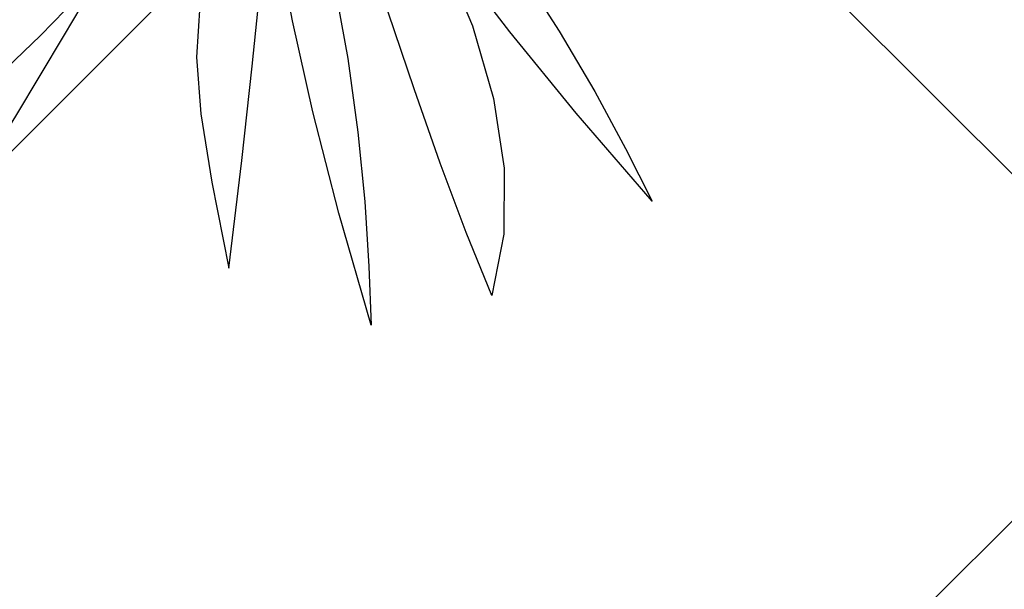
# Model space of a CAD drawing. Units: inches. Extents: x 3590 to 5167, y 65 to 1917.
# Tile 50 of 100: x 4947.17 to 4967.82, y 1503.63 to 1515.58. Entities that reach past the tile are written whole.
import ezdxf

# ---------------------------------------------------------------- set-up
doc = ezdxf.new("R2010")
doc.units = ezdxf.units.IN
doc.layers.add('A-FLOR-PATT', color=8, linetype='Continuous', lineweight=13)
doc.layers.add('L-PLNT', color=94, linetype='Continuous', lineweight=18)
doc.layers.add('DIENHOA', color=3, linetype='Continuous')

# ---------------------------------------------------------------- blocks, each defined once
blk = doc.blocks.new('Cay03_mb')
at = {"layer": 'DIENHOA'}
for p, q in [((135.85, -204.28), (162.8, -268.28)), ((-162.07, -230.91), (-206.29, -276.49)), ((113.06, -322.16), (90.79, -256.57)), ((162.8, -268.28), (180.96, -330.4)), ((-206.29, -276.49), (-249.56, -317.79)), ((135.38, -385.56), (113.06, -322.16)), ((180.96, -330.4), (190.01, -389.96)), ((157.6, -444.99), (135.38, -385.56)), ((190.01, -389.96), (189.65, -446.27)), ((179.55, -498.66), (157.6, -444.99)), ((189.65, -446.27), (179.55, -498.66))]:
    blk.add_line(p, q, dxfattribs=at)
for points in [[(23.69, -5.44), (-13.63, -87.94), (-41.14, -152.63), (-59.64, -205.04), (-69.94, -250.66), (-72.84, -295), (-69.17, -343.58), (-59.73, -401.89), (-45.32, -475.45)], [(-45.32, -475.45), (-34.09, -383.24), (-25.4, -302.82), (-18.34, -233.08), (-12.02, -172.9), (-5.55, -121.16), (1.96, -76.75), (11.41, -38.55), (23.69, -5.44)], [(316.49, -418.14), (251.44, -342.76), (194.84, -273.28), (146.52, -210.16), (106.33, -153.83), (74.11, -104.75), (49.71, -63.36), (32.95, -30.11), (23.69, -5.44)], [(23.69, -5.44), (74.94, -57.08), (121.78, -110.58), (164.32, -165.02), (202.67, -219.43), (236.95, -272.89), (267.27, -324.46), (293.75, -373.19), (316.49, -418.14)], [(-276.22, -424.43), (-227.35, -345.43), (-185.71, -276.08), (-150.05, -215.74), (-119.06, -163.76), (-91.49, -119.51), (-66.04, -82.35), (-41.43, -51.64), (-16.39, -26.73)], [(76.25, -524.2), (48.83, -428.48), (26.6, -341.67), (9.22, -264.1), (-3.63, -196.11), (-12.28, -138.04), (-17.07, -90.23), (-18.33, -53.01), (-16.39, -26.73)], [(-16.39, -26.73), (8.47, -95.11), (28.54, -163.33), (44.32, -230.59), (56.3, -296.08), (64.99, -358.99), (70.88, -418.52), (74.46, -473.86), (76.25, -524.2)]]:
    blk.add_lwpolyline(points, dxfattribs=at)

msp = doc.modelspace()

# ---------------------------------------------------------------- hatches: boundary and pattern name
at = {"layer": 'A-FLOR-PATT', "transparency": 33554687}
h = msp.add_hatch(dxfattribs=at)
h.set_pattern_fill('AR-HBONE', color=256, scale=0.2)
h.set_pattern_definition([(45, (-588.972, 0), (0, 28.73682), [60.96, -20.32]), (135, (-574.604, 14.368), (3e-15, 28.73682), [60.96, -20.32])])
h.paths.add_polyline_path([(5071.274, 1796.999), (4933.274, 1796.999), (4933.274, 1753.999), (4962.774, 1753.999, -0.414214), (4928.774, 1719.999), (4933.274, 1718.999), (4933.274, 1334.999), (5071.274, 1334.999)])
h.paths.add_polyline_path([(4951.78, 1521.077), (4951.715, 1521.04), (4951.563, 1520.895)], flags=16)
h.paths.add_polyline_path([(4952.267, 1521.376), (4952.198, 1521.371), (4952.198, 1521.356)], flags=0)
h.paths.add_polyline_path([(4967.051, 1529.728), (4965.231, 1528.694), (4963.411, 1527.714), (4961.756, 1526.851), (4963.589, 1527.449), (4964.036, 1527.478), (4962.975, 1527.249), (4961.76, 1526.852), (4959.792, 1525.834), (4958.005, 1524.895), (4956.24, 1523.93), (4954.504, 1522.919), (4954.129, 1522.682), (4953.361, 1521.997), (4953.366, 1521.998), (4953.605, 1522.064), (4955.106, 1522.761), (4956.921, 1523.434), (4958.678, 1523.915), (4960.358, 1524.2), (4961.945, 1524.286), (4964.171, 1524.108), (4965.958, 1523.309), (4963.863, 1522.976), (4965.187, 1522.499), (4963.366, 1522.497), (4961.545, 1522.487), (4959.764, 1522.461), (4958.304, 1522.419), (4957.974, 1522.388), (4956.307, 1522.232), (4954.718, 1522.071), (4953.251, 1521.899), (4953.525, 1521.623), (4954.331, 1521.379), (4956.243, 1521.23), (4958.039, 1520.93), (4959.684, 1520.483), (4961.16, 1519.896), (4963.107, 1518.8), (4964.393, 1517.325), (4962.973, 1517.726), (4964.558, 1516.661), (4965.407, 1515.708), (4963.507, 1516.322), (4961.68, 1517.005), (4959.935, 1517.745), (4958.282, 1518.528), (4956.732, 1519.343), (4955.295, 1520.175), (4954.672, 1520.572), (4954.513, 1520.627), (4955.658, 1519.318), (4956.703, 1517.982), (4957.644, 1516.647), (4958.485, 1515.334), (4959.55, 1513.524), (4960.438, 1511.769), (4958.841, 1513.62), (4957.452, 1515.325), (4955.819, 1517.459), (4956.665, 1515.448), (4957.111, 1513.923), (4957.447, 1511.714), (4957.076, 1509.793), (4956.538, 1511.11), (4955.992, 1512.569), (4955.444, 1514.125), (4954.898, 1515.735), (4954.357, 1517.356), (4953.824, 1518.943), (4953.305, 1520.452), (4953.065, 1521.116), (4952.971, 1521.146), (4952.949, 1521.086), (4952.73, 1520.199), (4953.37, 1518.024), (4953.757, 1516.373), (4954.051, 1514.765), (4954.264, 1513.221), (4954.471, 1511.131), (4954.497, 1510.402), (4954.409, 1511.76), (4954.264, 1513.221), (4954.051, 1514.765), (4953.757, 1516.373), (4953.37, 1518.024), (4952.877, 1519.698), (4952.716, 1520.141), (4952.533, 1519.059), (4952.374, 1517.789), (4952.219, 1516.312), (4952.046, 1514.6), (4951.833, 1512.626), (4951.557, 1510.363), (4951.203, 1512.168), (4950.852, 1514.339), (4950.985, 1516.376), (4951.66, 1518.286), (4952.593, 1520.481), (4952.357, 1521.13), (4951.855, 1520.328), (4950.839, 1518.908), (4949.777, 1517.587), (4948.916, 1516.617), (4948.111, 1515.256), (4947.089, 1513.554), (4945.889, 1511.615), (4946.326, 1513.402), (4946.562, 1514.249), (4945.528, 1513.327), (4944.581, 1512.531), (4946.018, 1514.508), (4947.204, 1516.048), (4947.893, 1517.313), (4949.307, 1518.764), (4950.414, 1519.767), (4950.451, 1519.806), (4952.267, 1521.376), (4951.645, 1521.493), (4950.404, 1521.18), (4948.044, 1520.359), (4946.119, 1519.452), (4944.572, 1518.475), (4943.35, 1517.443), (4941.997, 1515.92), (4941.661, 1515.275), (4942.813, 1516.99), (4944.572, 1518.475), (4946.119, 1519.452), (4948.044, 1520.359), (4950.404, 1521.18), (4951.645, 1521.493), (4949.647, 1521.868), (4948.6, 1521.756), (4947.126, 1521.57), (4945.42, 1521.348), (4943.45, 1521.105), (4941.183, 1520.856), (4942.86, 1521.613), (4943.873, 1522.03), (4942.952, 1521.909), (4941.41, 1521.485), (4939.543, 1520.67), (4938.968, 1520.226), (4940.733, 1521.299), (4942.952, 1521.909), (4943.702, 1522.008), (4945.894, 1522.7), (4947.565, 1522.714), (4948.921, 1522.566), (4951.131, 1522.183), (4950.971, 1522.297), (4948.129, 1523.006), (4946.035, 1523.707), (4944.232, 1524.521), (4942.707, 1525.461), (4941.444, 1526.537), (4940.43, 1527.761), (4939.649, 1529.143), (4941.421, 1528.122), (4943.147, 1527.132), (4944.841, 1526.175), (4946.514, 1525.25), (4948.179, 1524.359), (4948.365, 1524.263), (4946.475, 1526.045), (4945.181, 1527.54), (4944.19, 1529.033), (4943.496, 1530.54), (4943.278, 1531.36), (4942.498, 1531.919), (4943.114, 1531.762), (4942.959, 1533.659), (4944.14, 1531.989), (4944.612, 1531.323), (4946.202, 1530.463), (4947.486, 1529.509), (4948.79, 1528.226), (4950.368, 1526.237), (4949.485, 1528.155), (4948.851, 1530.123), (4948.491, 1532.041), (4948.381, 1533.918), (4948.501, 1535.76), (4948.827, 1537.573), (4949.418, 1535.565), (4949.957, 1533.569), (4950.464, 1531.586), (4950.961, 1529.617), (4951.391, 1527.954), (4951.724, 1530.687), (4952.201, 1532.58), (4952.889, 1534.33), (4953.77, 1535.951), (4954.827, 1537.46), (4954.521, 1535.39), (4954.273, 1533.937), (4955.58, 1535.663), (4956.748, 1536.739), (4956.159, 1534.78), (4955.589, 1532.873), (4955.043, 1531.006), (4954.525, 1529.166), (4954.038, 1527.341), (4953.638, 1525.733), (4953.611, 1525.586), (4953.398, 1524.166), (4953.382, 1524.009), (4954.07, 1525.476), (4954.912, 1527.022), (4956.136, 1528.894), (4957.847, 1530.577), (4959.376, 1531.54), (4958.256, 1530.104), (4957.143, 1528.663), (4956.066, 1527.243), (4955.056, 1525.871), (4954.141, 1524.571), (4953.352, 1523.372), (4953.311, 1523.303), (4953.273, 1522.925), (4953.261, 1522.382), (4954.103, 1523.373), (4954.63, 1524.284), (4955.961, 1526.358), (4957.23, 1528.13), (4958.421, 1529.609), (4960.037, 1531.368), (4961.374, 1532.375), (4962.101, 1532.77), (4961.07, 1531.061), (4959.987, 1529.438), (4958.869, 1527.908), (4958.15, 1527.007), (4959.803, 1528.003), (4961.589, 1528.793), (4963.391, 1529.328), (4965.211, 1529.632)], flags=16)
h.paths.add_polyline_path([(4962.944, 1523.182), (4961.107, 1523.422), (4960.392, 1523.362), (4962.35, 1523.331)], flags=0)
h.paths.add_polyline_path([(5049.541, 1584.551), (5049.476, 1584.515), (5049.325, 1584.37)], flags=16)
h.paths.add_polyline_path([(5050.028, 1584.851), (5049.959, 1584.845), (5049.959, 1584.83)], flags=0)
h.paths.add_polyline_path([(5042.333, 1581.949), (5043.88, 1582.926), (5045.806, 1583.833), (5048.165, 1584.654), (5049.406, 1584.967), (5047.408, 1585.342), (5046.361, 1585.231), (5044.888, 1585.044), (5043.181, 1584.822), (5041.211, 1584.579), (5038.944, 1584.33), (5040.622, 1585.087), (5041.634, 1585.504), (5040.713, 1585.383), (5039.171, 1584.959), (5037.304, 1584.144), (5036.729, 1583.7), (5038.494, 1584.773), (5040.713, 1585.383), (5041.463, 1585.482), (5043.655, 1586.174), (5045.326, 1586.188), (5046.682, 1586.04), (5048.893, 1585.657), (5048.732, 1585.771), (5045.891, 1586.48), (5043.796, 1587.181), (5041.994, 1587.996), (5040.468, 1588.935), (5039.205, 1590.011), (5038.191, 1591.235), (5037.41, 1592.617), (5039.182, 1591.596), (5040.909, 1590.607), (5042.602, 1589.649), (5044.275, 1588.724), (5045.94, 1587.833), (5046.126, 1587.738), (5044.237, 1589.519), (5042.942, 1591.015), (5041.952, 1592.508), (5041.257, 1594.014), (5041.039, 1594.834), (5040.26, 1595.393), (5040.875, 1595.237), (5040.721, 1597.133), (5041.901, 1595.463), (5042.373, 1594.798), (5043.963, 1593.938), (5045.247, 1592.983), (5046.552, 1591.701), (5048.129, 1589.712), (5047.247, 1591.63), (5046.613, 1593.597), (5046.252, 1595.515), (5046.142, 1597.392), (5046.262, 1599.234), (5046.588, 1601.047), (5047.179, 1599.039), (5047.718, 1597.043), (5048.225, 1595.06), (5048.722, 1593.091), (5049.152, 1591.429), (5049.485, 1594.161), (5049.962, 1596.054), (5050.65, 1597.804), (5051.532, 1599.425), (5052.589, 1600.934), (5052.283, 1598.864), (5052.034, 1597.411), (5053.341, 1599.137), (5054.509, 1600.213), (5053.92, 1598.254), (5053.35, 1596.348), (5052.805, 1594.48), (5052.286, 1592.64), (5051.799, 1590.815), (5051.4, 1589.207), (5051.373, 1589.06), (5051.159, 1587.64), (5051.143, 1587.483), (5051.831, 1588.95), (5052.673, 1590.496), (5053.898, 1592.368), (5055.608, 1594.051), (5057.137, 1595.014), (5056.017, 1593.578), (5054.904, 1592.137), (5053.828, 1590.717), (5052.817, 1589.345), (5051.902, 1588.046), (5051.113, 1586.846), (5051.072, 1586.777), (5051.034, 1586.399), (5051.022, 1585.856), (5051.864, 1586.847), (5052.391, 1587.758), (5053.723, 1589.832), (5054.991, 1591.604), (5056.182, 1593.083), (5057.798, 1594.842), (5059.135, 1595.849), (5059.863, 1596.244), (5058.831, 1594.535), (5057.749, 1592.912), (5056.63, 1591.382), (5055.912, 1590.482), (5057.564, 1591.477), (5059.35, 1592.267), (5061.152, 1592.802), (5062.972, 1593.106), (5064.812, 1593.203), (5062.992, 1592.169), (5061.172, 1591.188), (5059.518, 1590.325), (5061.35, 1590.924), (5061.797, 1590.952), (5060.737, 1590.723), (5059.521, 1590.326), (5057.553, 1589.308), (5055.766, 1588.369), (5054.002, 1587.404), (5052.265, 1586.393), (5051.891, 1586.156), (5051.122, 1585.471), (5051.127, 1585.472), (5051.366, 1585.538), (5052.867, 1586.235), (5054.682, 1586.908), (5056.439, 1587.389), (5058.12, 1587.675), (5059.706, 1587.76), (5061.933, 1587.583), (5063.719, 1586.783), (5061.624, 1586.45), (5062.949, 1585.973), (5061.127, 1585.971), (5059.307, 1585.961), (5057.525, 1585.935), (5056.065, 1585.893), (5055.735, 1585.862), (5054.068, 1585.707), (5052.479, 1585.546), (5051.012, 1585.373), (5051.286, 1585.097), (5052.092, 1584.853), (5054.004, 1584.704), (5055.8, 1584.404), (5057.446, 1583.958), (5058.921, 1583.37), (5060.868, 1582.274), (5062.154, 1580.799), (5060.734, 1581.2), (5062.32, 1580.135), (5063.168, 1579.182), (5061.269, 1579.796), (5059.441, 1580.479), (5057.696, 1581.219), (5056.043, 1582.003), (5054.493, 1582.817), (5053.057, 1583.649), (5052.433, 1584.047), (5052.274, 1584.101), (5053.42, 1582.793), (5054.464, 1581.457), (5055.405, 1580.121), (5056.247, 1578.809), (5057.311, 1576.998), (5058.199, 1575.244), (5056.602, 1577.094), (5055.213, 1578.799), (5053.58, 1580.933), (5054.427, 1578.922), (5054.872, 1577.397), (5055.208, 1575.189), (5054.838, 1573.267), (5054.299, 1574.584), (5053.754, 1576.043), (5053.206, 1577.599), (5052.659, 1579.209), (5052.118, 1580.83), (5051.585, 1582.417), (5051.066, 1583.927), (5050.826, 1584.59), (5050.733, 1584.62), (5050.711, 1584.561), (5050.491, 1583.673), (5051.131, 1581.498), (5051.518, 1579.847), (5051.813, 1578.24), (5052.026, 1576.695), (5052.233, 1574.605), (5052.258, 1573.876), (5052.17, 1575.234), (5052.026, 1576.695), (5051.813, 1578.24), (5051.518, 1579.847), (5051.131, 1581.498), (5050.638, 1583.172), (5050.477, 1583.615), (5050.294, 1582.533), (5050.136, 1581.263), (5049.981, 1579.786), (5049.807, 1578.074), (5049.594, 1576.1), (5049.318, 1573.837), (5048.965, 1575.642), (5048.613, 1577.813), (5048.747, 1579.85), (5049.421, 1581.76), (5050.354, 1583.955), (5050.118, 1584.604), (5049.616, 1583.802), (5048.6, 1582.382), (5047.538, 1581.061), (5046.677, 1580.091), (5045.872, 1578.73), (5044.85, 1577.028), (5043.651, 1575.089), (5044.087, 1576.877), (5044.324, 1577.723), (5043.289, 1576.801), (5042.342, 1576.005), (5043.779, 1577.982), (5044.966, 1579.522), (5045.655, 1580.787), (5047.068, 1582.239), (5048.175, 1583.241), (5048.213, 1583.28), (5050.028, 1584.851), (5049.406, 1584.967), (5048.165, 1584.654), (5045.806, 1583.833), (5043.88, 1582.926), (5042.333, 1581.949), (5041.111, 1580.917), (5039.758, 1579.394), (5039.423, 1578.749), (5040.575, 1580.464)], flags=16)
h.paths.add_polyline_path([(4954.799, 1533.12), (4954.262, 1532.079), (4953.831, 1530.935), (4953.505, 1529.636), (4953.283, 1528.133), (4953.167, 1526.376), (4953.156, 1524.315), (4953.277, 1521.236), (4952.802, 1521.842), (4951.557, 1521.998), (4950.976, 1521.961), (4952.661, 1521.941), (4952.802, 1521.842), (4953.152, 1523.593), (4953.167, 1526.376), (4953.283, 1528.133), (4953.609, 1530.346), (4954.456, 1532.592)], flags=0)
h.paths.add_polyline_path([(5050.563, 1585.316), (5049.318, 1585.472), (5048.737, 1585.435), (5050.422, 1585.415), (5050.563, 1585.316), (5050.914, 1587.067), (5050.928, 1589.851), (5051.045, 1591.607), (5051.371, 1593.82), (5052.217, 1596.066), (5052.56, 1596.594), (5052.024, 1595.554), (5051.592, 1594.409), (5051.266, 1593.11), (5051.045, 1591.607), (5050.928, 1589.851), (5050.918, 1587.789), (5051.038, 1584.71)], flags=0)
h.paths.add_polyline_path([(5058.153, 1586.836), (5060.111, 1586.805), (5060.705, 1586.656), (5058.868, 1586.896)], flags=0)
h.paths.add_polyline_path([(5049.541, 1430.936), (5049.476, 1430.9), (5049.325, 1430.755)], flags=16)
h.paths.add_polyline_path([(5050.028, 1431.236), (5049.959, 1431.231), (5049.959, 1431.215)], flags=0)
h.paths.add_polyline_path([(5046.588, 1447.432), (5047.179, 1445.425), (5047.718, 1443.429), (5048.225, 1441.446), (5048.722, 1439.476), (5049.152, 1437.814), (5049.485, 1440.546), (5049.962, 1442.439), (5050.65, 1444.189), (5051.532, 1445.811), (5052.589, 1447.319), (5052.283, 1445.249), (5052.034, 1443.796), (5053.341, 1445.522), (5054.509, 1446.598), (5053.92, 1444.64), (5053.35, 1442.733), (5052.805, 1440.865), (5052.286, 1439.025), (5051.799, 1437.201), (5051.4, 1435.592), (5051.373, 1435.445), (5051.159, 1434.025), (5051.143, 1433.868), (5051.831, 1435.335), (5052.673, 1436.881), (5053.898, 1438.753), (5055.608, 1440.436), (5057.137, 1441.4), (5056.017, 1439.963), (5054.904, 1438.522), (5053.828, 1437.102), (5052.817, 1435.73), (5051.902, 1434.431), (5051.113, 1433.231), (5051.072, 1433.162), (5051.034, 1432.784), (5051.022, 1432.242), (5051.864, 1433.232), (5052.391, 1434.143), (5053.723, 1436.217), (5054.991, 1437.989), (5056.182, 1439.468), (5057.798, 1441.227), (5059.135, 1442.235), (5059.863, 1442.629), (5058.831, 1440.921), (5057.749, 1439.298), (5056.63, 1437.767), (5055.912, 1436.867), (5057.564, 1437.863), (5059.35, 1438.652), (5061.152, 1439.187), (5062.972, 1439.491), (5064.812, 1439.588), (5062.992, 1438.554), (5061.172, 1437.573), (5059.518, 1436.71), (5061.35, 1437.309), (5061.797, 1437.337), (5060.737, 1437.108), (5059.521, 1436.711), (5057.553, 1435.693), (5055.766, 1434.754), (5054.002, 1433.789), (5052.265, 1432.778), (5051.891, 1432.541), (5051.122, 1431.856), (5051.127, 1431.857), (5051.366, 1431.923), (5052.867, 1432.62), (5054.682, 1433.293), (5056.439, 1433.775), (5058.12, 1434.06), (5059.706, 1434.145), (5061.933, 1433.968), (5063.719, 1433.168), (5061.624, 1432.835), (5062.949, 1432.358), (5061.127, 1432.357), (5059.307, 1432.346), (5057.525, 1432.32), (5056.065, 1432.278), (5055.735, 1432.248), (5054.068, 1432.092), (5052.479, 1431.931), (5051.012, 1431.759), (5051.286, 1431.482), (5052.092, 1431.238), (5054.004, 1431.089), (5055.8, 1430.789), (5057.446, 1430.343), (5058.921, 1429.755), (5060.868, 1428.66), (5062.154, 1427.185), (5060.734, 1427.585), (5062.32, 1426.52), (5063.168, 1425.567), (5061.269, 1426.181), (5059.441, 1426.865), (5057.696, 1427.604), (5056.043, 1428.388), (5054.493, 1429.202), (5053.057, 1430.034), (5052.433, 1430.432), (5052.274, 1430.487), (5053.42, 1429.178), (5054.464, 1427.842), (5055.405, 1426.506), (5056.247, 1425.194), (5057.311, 1423.383), (5058.199, 1421.629), (5056.602, 1423.479), (5055.213, 1425.184), (5053.58, 1427.318), (5054.427, 1425.307), (5054.872, 1423.782), (5055.208, 1421.574), (5054.838, 1419.652), (5054.299, 1420.97), (5053.754, 1422.428), (5053.206, 1423.984), (5052.659, 1425.595), (5052.118, 1427.215), (5051.585, 1428.802), (5051.066, 1430.312), (5050.826, 1430.975), (5050.733, 1431.005), (5050.711, 1430.946), (5050.491, 1430.058), (5051.131, 1427.883), (5051.518, 1426.232), (5051.813, 1424.625), (5052.026, 1423.081), (5052.233, 1420.991), (5052.258, 1420.261), (5052.17, 1421.619), (5052.026, 1423.081), (5051.813, 1424.625), (5051.518, 1426.232), (5051.131, 1427.883), (5050.638, 1429.558), (5050.477, 1430.001), (5050.294, 1428.918), (5050.136, 1427.648), (5049.981, 1426.171), (5049.807, 1424.459), (5049.594, 1422.485), (5049.318, 1420.222), (5048.965, 1422.028), (5048.613, 1424.199), (5048.747, 1426.235), (5049.421, 1428.146), (5050.354, 1430.34), (5050.118, 1430.989), (5049.616, 1430.187), (5048.6, 1428.768), (5047.538, 1427.446), (5046.677, 1426.477), (5045.872, 1425.116), (5044.85, 1423.413), (5043.651, 1421.474), (5044.087, 1423.262), (5044.324, 1424.109), (5043.289, 1423.186), (5042.342, 1422.391), (5043.779, 1424.368), (5044.966, 1425.907), (5045.655, 1427.173), (5047.068, 1428.624), (5048.175, 1429.627), (5048.213, 1429.666), (5050.028, 1431.236), (5049.406, 1431.353), (5048.165, 1431.039), (5045.806, 1430.218), (5043.88, 1429.311), (5042.333, 1428.334), (5041.111, 1427.302), (5039.758, 1425.779), (5039.423, 1425.134), (5040.575, 1426.849), (5042.333, 1428.334), (5043.88, 1429.311), (5045.806, 1430.218), (5048.165, 1431.039), (5049.406, 1431.353), (5047.408, 1431.727), (5046.361, 1431.616), (5044.888, 1431.429), (5043.181, 1431.207), (5041.211, 1430.964), (5038.944, 1430.715), (5040.622, 1431.472), (5041.634, 1431.89), (5040.713, 1431.769), (5039.171, 1431.345), (5037.304, 1430.53), (5036.729, 1430.085), (5038.494, 1431.158), (5040.713, 1431.769), (5041.463, 1431.867), (5043.655, 1432.559), (5045.326, 1432.573), (5046.682, 1432.425), (5048.893, 1432.042), (5048.732, 1432.156), (5045.891, 1432.865), (5043.796, 1433.566), (5041.994, 1434.381), (5040.468, 1435.321), (5039.205, 1436.396), (5038.191, 1437.62), (5037.41, 1439.002), (5039.182, 1437.982), (5040.909, 1436.992), (5042.602, 1436.034), (5044.275, 1435.109), (5045.94, 1434.218), (5046.126, 1434.123), (5044.237, 1435.904), (5042.942, 1437.4), (5041.952, 1438.893), (5041.257, 1440.399), (5041.039, 1441.219), (5040.26, 1441.778), (5040.875, 1441.622), (5040.721, 1443.518), (5041.901, 1441.848), (5042.373, 1441.183), (5043.963, 1440.323), (5045.247, 1439.369), (5046.552, 1438.086), (5048.129, 1436.097), (5047.247, 1438.015), (5046.613, 1439.982), (5046.252, 1441.901), (5046.142, 1443.778), (5046.262, 1445.619)], flags=16)
h.paths.add_polyline_path([(5052.382, 1444.255), (5051.623, 1442.78), (5052.024, 1441.939), (5052.56, 1442.98)], flags=0)
h.paths.add_polyline_path([(5050.563, 1431.701), (5049.318, 1431.857), (5048.737, 1431.821), (5050.422, 1431.8)], flags=0)
h.paths.add_polyline_path([(5058.153, 1433.221), (5060.111, 1433.19), (5060.705, 1433.041), (5058.868, 1433.281)], flags=0)
h.paths.add_polyline_path([(5049.541, 1352.285), (5049.476, 1352.249), (5049.325, 1352.104)], flags=16)
h.paths.add_polyline_path([(5050.028, 1352.585), (5049.959, 1352.58), (5049.959, 1352.564)], flags=0)
h.paths.add_polyline_path([(5046.588, 1368.781), (5047.179, 1366.774), (5047.718, 1364.778), (5048.225, 1362.795), (5048.722, 1360.825), (5049.152, 1359.163), (5049.485, 1361.896), (5049.962, 1363.789), (5050.65, 1365.538), (5051.532, 1367.16), (5052.589, 1368.669), (5052.283, 1366.598), (5052.034, 1365.145), (5053.341, 1366.871), (5054.509, 1367.947), (5053.92, 1365.989), (5053.35, 1364.082), (5052.805, 1362.214), (5052.286, 1360.374), (5051.799, 1358.55), (5051.4, 1356.942), (5051.373, 1356.794), (5051.159, 1355.374), (5051.143, 1355.218), (5051.831, 1356.684), (5052.673, 1358.23), (5053.898, 1360.102), (5055.608, 1361.786), (5057.137, 1362.749), (5056.017, 1361.313), (5054.904, 1359.872), (5053.828, 1358.452), (5052.817, 1357.079), (5051.902, 1355.78), (5051.113, 1354.581), (5051.072, 1354.512), (5051.034, 1354.133), (5051.022, 1353.591), (5051.864, 1354.581), (5052.391, 1355.492), (5053.723, 1357.566), (5054.991, 1359.338), (5056.182, 1360.817), (5057.798, 1362.577), (5059.135, 1363.584), (5059.863, 1363.979), (5058.831, 1362.27), (5057.749, 1360.647), (5056.63, 1359.117), (5055.912, 1358.216), (5057.564, 1359.212), (5059.35, 1360.001), (5061.152, 1360.536), (5062.972, 1360.841), (5064.812, 1360.937), (5062.992, 1359.903), (5061.172, 1358.923), (5059.518, 1358.059), (5061.35, 1358.658), (5061.797, 1358.687), (5060.737, 1358.458), (5059.521, 1358.061), (5057.553, 1357.043), (5055.766, 1356.103), (5054.002, 1355.138), (5052.265, 1354.127), (5051.891, 1353.89), (5051.122, 1353.206), (5051.127, 1353.206), (5051.366, 1353.272), (5052.867, 1353.969), (5054.682, 1354.643), (5056.439, 1355.124), (5058.12, 1355.409), (5059.706, 1355.495), (5061.933, 1355.317), (5063.719, 1354.518), (5061.624, 1354.184), (5062.949, 1353.708), (5061.127, 1353.706), (5059.307, 1353.695), (5057.525, 1353.669), (5056.065, 1353.627), (5055.735, 1353.597), (5054.068, 1353.441), (5052.479, 1353.28), (5051.012, 1353.108), (5051.286, 1352.831), (5052.092, 1352.587), (5054.004, 1352.439), (5055.8, 1352.138), (5057.446, 1351.692), (5058.921, 1351.104), (5060.868, 1350.009), (5062.154, 1348.534), (5060.734, 1348.935), (5062.32, 1347.869), (5063.168, 1346.916), (5061.269, 1347.53), (5059.441, 1348.214), (5057.696, 1348.954), (5056.043, 1349.737), (5054.493, 1350.551), (5053.057, 1351.383), (5052.433, 1351.781), (5052.274, 1351.836), (5053.42, 1350.527), (5054.464, 1349.191), (5055.405, 1347.855), (5056.247, 1346.543), (5057.311, 1344.733), (5058.199, 1342.978), (5056.602, 1344.828), (5055.213, 1346.534), (5053.58, 1348.667), (5054.427, 1346.656), (5054.872, 1345.132), (5055.208, 1342.923), (5054.838, 1341.002), (5054.299, 1342.319), (5053.754, 1343.778), (5053.206, 1345.334), (5052.659, 1346.944), (5052.118, 1348.564), (5051.585, 1350.151), (5051.066, 1351.661), (5050.826, 1352.324), (5050.733, 1352.355), (5050.711, 1352.295), (5050.491, 1351.408), (5051.131, 1349.232), (5051.518, 1347.581), (5051.813, 1345.974), (5052.026, 1344.43), (5052.233, 1342.34), (5052.258, 1341.61), (5052.17, 1342.969), (5052.026, 1344.43), (5051.813, 1345.974), (5051.518, 1347.581), (5051.131, 1349.232), (5050.638, 1350.907), (5050.477, 1351.35), (5050.294, 1350.267), (5050.136, 1348.997), (5049.981, 1347.52), (5049.807, 1345.809), (5049.594, 1343.835), (5049.318, 1341.571), (5048.965, 1343.377), (5048.613, 1345.548), (5048.747, 1347.585), (5049.421, 1349.495), (5050.354, 1351.689), (5050.118, 1352.339), (5049.616, 1351.536), (5048.6, 1350.117), (5047.538, 1348.795), (5046.677, 1347.826), (5045.872, 1346.465), (5044.85, 1344.763), (5043.651, 1342.824), (5044.087, 1344.611), (5044.324, 1345.458), (5043.289, 1344.535), (5042.342, 1343.74), (5043.779, 1345.717), (5044.966, 1347.256), (5045.655, 1348.522), (5047.068, 1349.973), (5048.175, 1350.976), (5048.213, 1351.015), (5050.028, 1352.585), (5049.406, 1352.702), (5048.165, 1352.388), (5045.806, 1351.567), (5043.88, 1350.661), (5042.333, 1349.683), (5041.111, 1348.651), (5039.758, 1347.128), (5039.423, 1346.483), (5040.575, 1348.198), (5042.333, 1349.683), (5043.88, 1350.661), (5045.806, 1351.567), (5048.165, 1352.388), (5049.406, 1352.702), (5047.408, 1353.076), (5046.361, 1352.965), (5044.888, 1352.779), (5043.181, 1352.556), (5041.211, 1352.313), (5038.944, 1352.065), (5040.622, 1352.821), (5041.634, 1353.239), (5040.713, 1353.118), (5039.171, 1352.694), (5037.304, 1351.879), (5036.729, 1351.434), (5038.494, 1352.508), (5040.713, 1353.118), (5041.463, 1353.216), (5043.655, 1353.909), (5045.326, 1353.923), (5046.682, 1353.774), (5048.893, 1353.391), (5048.732, 1353.506), (5045.891, 1354.214), (5043.796, 1354.915), (5041.994, 1355.73), (5040.468, 1356.67), (5039.205, 1357.746), (5038.191, 1358.969), (5037.41, 1360.352), (5039.182, 1359.331), (5040.909, 1358.341), (5042.602, 1357.383), (5044.275, 1356.458), (5045.94, 1355.567), (5046.126, 1355.472), (5044.237, 1357.253), (5042.942, 1358.749), (5041.952, 1360.242), (5041.257, 1361.748), (5041.039, 1362.568), (5040.26, 1363.128), (5040.875, 1362.971), (5040.721, 1364.867), (5041.901, 1363.197), (5042.373, 1362.532), (5043.963, 1361.672), (5045.247, 1360.718), (5046.552, 1359.435), (5048.129, 1357.446), (5047.247, 1359.364), (5046.613, 1361.331), (5046.252, 1363.25), (5046.142, 1365.127), (5046.262, 1366.969)], flags=16)
h.paths.add_polyline_path([(5052.382, 1365.604), (5051.623, 1364.129), (5052.024, 1363.288), (5052.56, 1364.329)], flags=0)
h.paths.add_polyline_path([(4951.78, 1698.041), (4951.715, 1698.005), (4951.563, 1697.859)], flags=16)
h.paths.add_polyline_path([(4952.267, 1698.341), (4952.198, 1698.335), (4952.198, 1698.32)], flags=0)
h.paths.add_polyline_path([(4957.076, 1686.757), (4956.538, 1688.074), (4955.992, 1689.533), (4955.444, 1691.089), (4954.898, 1692.699), (4954.357, 1694.32), (4953.824, 1695.907), (4953.305, 1697.417), (4953.065, 1698.08), (4952.971, 1698.11), (4952.949, 1698.051), (4952.73, 1697.163), (4953.37, 1694.988), (4953.757, 1693.337), (4954.051, 1691.729), (4954.264, 1690.185), (4954.471, 1688.095), (4954.497, 1687.366), (4954.409, 1688.724), (4954.264, 1690.185), (4954.051, 1691.729), (4953.757, 1693.337), (4953.37, 1694.988), (4952.877, 1696.662), (4952.716, 1697.105), (4952.533, 1696.023), (4952.374, 1694.753), (4952.219, 1693.276), (4952.046, 1691.564), (4951.833, 1689.59), (4951.557, 1687.327), (4951.203, 1689.132), (4950.852, 1691.303), (4950.985, 1693.34), (4951.66, 1695.25), (4952.593, 1697.445), (4952.357, 1698.094), (4951.855, 1697.292), (4950.839, 1695.872), (4949.777, 1694.551), (4948.916, 1693.581), (4948.111, 1692.22), (4947.089, 1690.518), (4945.889, 1688.579), (4946.326, 1690.366), (4946.562, 1691.213), (4945.528, 1690.291), (4944.581, 1689.495), (4946.018, 1691.472), (4947.204, 1693.012), (4947.893, 1694.277), (4949.307, 1695.729), (4950.414, 1696.731), (4950.451, 1696.77), (4952.267, 1698.341), (4951.645, 1698.457), (4950.404, 1698.144), (4948.044, 1697.323), (4946.119, 1696.416), (4944.572, 1695.439), (4943.35, 1694.407), (4941.997, 1692.884), (4941.661, 1692.239), (4942.813, 1693.954), (4944.572, 1695.439), (4946.119, 1696.416), (4948.044, 1697.323), (4950.404, 1698.144), (4951.645, 1698.457), (4949.647, 1698.832), (4948.6, 1698.72), (4947.126, 1698.534), (4945.42, 1698.312), (4943.45, 1698.069), (4941.183, 1697.82), (4942.86, 1698.577), (4943.873, 1698.994), (4942.952, 1698.873), (4941.41, 1698.449), (4939.543, 1697.634), (4938.968, 1697.19), (4940.733, 1698.263), (4942.952, 1698.873), (4943.702, 1698.972), (4945.894, 1699.664), (4947.565, 1699.678), (4948.921, 1699.53), (4951.131, 1699.147), (4950.971, 1699.261), (4948.129, 1699.97), (4946.035, 1700.671), (4944.232, 1701.486), (4942.707, 1702.425), (4941.444, 1703.501), (4940.43, 1704.725), (4939.649, 1706.107), (4941.421, 1705.086), (4943.147, 1704.097), (4944.841, 1703.139), (4946.514, 1702.214), (4948.179, 1701.323), (4948.365, 1701.227), (4946.475, 1703.009), (4945.181, 1704.505), (4944.19, 1705.997), (4943.496, 1707.504), (4943.278, 1708.324), (4942.498, 1708.883), (4943.114, 1708.727), (4942.959, 1710.623), (4944.14, 1708.953), (4944.612, 1708.287), (4946.202, 1707.428), (4947.486, 1706.473), (4948.79, 1705.191), (4950.368, 1703.202), (4949.485, 1705.12), (4948.851, 1707.087), (4948.491, 1709.005), (4948.381, 1710.882), (4948.501, 1712.724), (4948.827, 1714.537), (4949.418, 1712.529), (4949.957, 1710.533), (4950.464, 1708.55), (4950.961, 1706.581), (4951.391, 1704.919), (4951.724, 1707.651), (4952.201, 1709.544), (4952.889, 1711.294), (4953.77, 1712.915), (4954.827, 1714.424), (4954.521, 1712.354), (4954.273, 1710.901), (4955.58, 1712.627), (4956.748, 1713.703), (4956.159, 1711.744), (4955.589, 1709.837), (4955.043, 1707.97), (4954.525, 1706.13), (4954.038, 1704.305), (4953.638, 1702.697), (4953.611, 1702.55), (4953.398, 1701.13), (4953.382, 1700.973), (4954.07, 1702.44), (4954.912, 1703.986), (4956.136, 1705.858), (4957.847, 1707.541), (4959.376, 1708.504), (4958.256, 1707.068), (4957.143, 1705.627), (4956.066, 1704.207), (4955.056, 1702.835), (4954.141, 1701.536), (4953.352, 1700.336), (4953.311, 1700.267), (4953.273, 1699.889), (4953.261, 1699.346), (4954.103, 1700.337), (4954.63, 1701.248), (4955.961, 1703.322), (4957.23, 1705.094), (4958.421, 1706.573), (4960.037, 1708.332), (4961.374, 1709.339), (4962.101, 1709.734), (4961.07, 1708.025), (4959.987, 1706.402), (4958.869, 1704.872), (4958.15, 1703.972), (4959.803, 1704.967), (4961.589, 1705.757), (4963.391, 1706.292), (4965.211, 1706.596), (4967.051, 1706.692), (4965.231, 1705.659), (4963.411, 1704.678), (4961.756, 1703.815), (4963.589, 1704.413), (4964.036, 1704.442), (4962.975, 1704.213), (4961.76, 1703.816), (4959.792, 1702.798), (4958.005, 1701.859), (4956.24, 1700.894), (4954.504, 1699.883), (4954.129, 1699.646), (4953.361, 1698.961), (4953.366, 1698.962), (4953.605, 1699.028), (4955.106, 1699.725), (4956.921, 1700.398), (4958.678, 1700.879), (4960.358, 1701.164), (4961.945, 1701.25), (4964.171, 1701.073), (4965.958, 1700.273), (4963.863, 1699.94), (4965.187, 1699.463), (4963.366, 1699.461), (4961.545, 1699.451), (4959.764, 1699.425), (4958.304, 1699.383), (4957.974, 1699.352), (4956.307, 1699.197), (4954.718, 1699.036), (4953.251, 1698.863), (4953.525, 1698.587), (4954.331, 1698.343), (4956.243, 1698.194), (4958.039, 1697.894), (4959.684, 1697.447), (4961.16, 1696.86), (4963.107, 1695.764), (4964.393, 1694.289), (4962.973, 1694.69), (4964.558, 1693.625), (4965.407, 1692.672), (4963.507, 1693.286), (4961.68, 1693.969), (4959.935, 1694.709), (4958.282, 1695.492), (4956.732, 1696.307), (4955.295, 1697.139), (4954.672, 1697.536), (4954.513, 1697.591), (4955.658, 1696.282), (4956.703, 1694.946), (4957.644, 1693.611), (4958.485, 1692.298), (4959.55, 1690.488), (4960.438, 1688.733), (4958.841, 1690.584), (4957.452, 1692.289), (4955.819, 1694.423), (4956.665, 1692.412), (4957.111, 1690.887), (4957.447, 1688.678)], flags=16)
h.paths.add_polyline_path([(5050.563, 1353.05), (5049.318, 1353.207), (5048.737, 1353.17), (5050.422, 1353.15)], flags=0)
h.paths.add_polyline_path([(4951.78, 1351.486), (4951.715, 1351.45), (4951.563, 1351.305)], flags=16)
h.paths.add_polyline_path([(4952.267, 1351.786), (4952.198, 1351.78), (4952.198, 1351.765)], flags=0)
h.paths.add_polyline_path([(4954.827, 1367.869), (4954.521, 1365.799), (4954.273, 1364.346), (4955.58, 1366.072), (4956.748, 1367.148), (4956.159, 1365.19), (4955.589, 1363.283), (4955.043, 1361.415), (4954.525, 1359.575), (4954.038, 1357.751), (4953.638, 1356.142), (4953.611, 1355.995), (4953.398, 1354.575), (4953.382, 1354.418), (4954.07, 1355.885), (4954.912, 1357.431), (4956.136, 1359.303), (4957.847, 1360.986), (4959.376, 1361.95), (4958.256, 1360.513), (4957.143, 1359.072), (4956.066, 1357.652), (4955.056, 1356.28), (4954.141, 1354.981), (4953.352, 1353.781), (4953.311, 1353.712), (4953.273, 1353.334), (4953.261, 1352.792), (4954.103, 1353.782), (4954.63, 1354.693), (4955.961, 1356.767), (4957.23, 1358.539), (4958.421, 1360.018), (4960.037, 1361.777), (4961.374, 1362.785), (4962.101, 1363.179), (4961.07, 1361.471), (4959.987, 1359.848), (4958.869, 1358.317), (4958.15, 1357.417), (4959.803, 1358.413), (4961.589, 1359.202), (4963.391, 1359.737), (4965.211, 1360.041), (4967.051, 1360.138), (4965.231, 1359.104), (4963.411, 1358.123), (4961.756, 1357.26), (4963.589, 1357.859), (4964.036, 1357.887), (4962.975, 1357.658), (4961.76, 1357.261), (4959.792, 1356.243), (4958.005, 1355.304), (4956.24, 1354.339), (4954.504, 1353.328), (4954.129, 1353.091), (4953.361, 1352.406), (4953.366, 1352.407), (4953.605, 1352.473), (4955.106, 1353.17), (4956.921, 1353.843), (4958.678, 1354.325), (4960.358, 1354.61), (4961.945, 1354.695), (4964.171, 1354.518), (4965.958, 1353.718), (4963.863, 1353.385), (4965.187, 1352.908), (4963.366, 1352.907), (4961.545, 1352.896), (4959.764, 1352.87), (4958.304, 1352.828), (4957.974, 1352.798), (4956.307, 1352.642), (4954.718, 1352.481), (4953.251, 1352.309), (4953.525, 1352.032), (4954.331, 1351.788), (4956.243, 1351.639), (4958.039, 1351.339), (4959.684, 1350.893), (4961.16, 1350.305), (4963.107, 1349.21), (4964.393, 1347.735), (4962.973, 1348.135), (4964.558, 1347.07), (4965.407, 1346.117), (4963.507, 1346.731), (4961.68, 1347.414), (4959.935, 1348.154), (4958.282, 1348.938), (4956.732, 1349.752), (4955.295, 1350.584), (4954.672, 1350.982), (4954.513, 1351.036), (4955.658, 1349.728), (4956.703, 1348.392), (4957.644, 1347.056), (4958.485, 1345.744), (4959.55, 1343.933), (4960.438, 1342.179), (4958.841, 1344.029), (4957.452, 1345.734), (4955.819, 1347.868), (4956.665, 1345.857), (4957.111, 1344.332), (4957.447, 1342.124), (4957.076, 1340.202), (4956.538, 1341.52), (4955.992, 1342.978), (4955.444, 1344.534), (4954.898, 1346.145), (4954.357, 1347.765), (4953.824, 1349.352), (4953.305, 1350.862), (4953.065, 1351.525), (4952.971, 1351.555), (4952.949, 1351.496), (4952.73, 1350.608), (4953.37, 1348.433), (4953.757, 1346.782), (4954.051, 1345.175), (4954.264, 1343.631), (4954.471, 1341.541), (4954.497, 1340.811), (4954.409, 1342.169), (4954.264, 1343.631), (4954.051, 1345.175), (4953.757, 1346.782), (4953.37, 1348.433), (4952.877, 1350.108), (4952.716, 1350.551), (4952.533, 1349.468), (4952.374, 1348.198), (4952.219, 1346.721), (4952.046, 1345.009), (4951.833, 1343.035), (4951.557, 1340.772), (4951.203, 1342.578), (4950.852, 1344.749), (4950.985, 1346.785), (4951.66, 1348.696), (4952.593, 1350.89), (4952.357, 1351.539), (4951.855, 1350.737), (4950.839, 1349.318), (4949.777, 1347.996), (4948.916, 1347.027), (4948.111, 1345.665), (4947.089, 1343.963), (4945.889, 1342.024), (4946.326, 1343.812), (4946.562, 1344.659), (4945.528, 1343.736), (4944.581, 1342.941), (4946.018, 1344.918), (4947.204, 1346.457), (4947.893, 1347.723), (4949.307, 1349.174), (4950.414, 1350.177), (4950.451, 1350.216), (4952.267, 1351.786), (4951.645, 1351.903), (4950.404, 1351.589), (4948.044, 1350.768), (4946.119, 1349.861), (4944.572, 1348.884), (4943.35, 1347.852), (4941.997, 1346.329), (4941.661, 1345.684), (4942.813, 1347.399), (4944.572, 1348.884), (4946.119, 1349.861), (4948.044, 1350.768), (4950.404, 1351.589), (4951.645, 1351.903), (4949.647, 1352.277), (4948.6, 1352.166), (4947.126, 1351.979), (4945.42, 1351.757), (4943.45, 1351.514), (4941.183, 1351.265), (4942.86, 1352.022), (4943.873, 1352.44), (4942.952, 1352.319), (4941.41, 1351.895), (4939.543, 1351.08), (4938.968, 1350.635), (4940.733, 1351.708), (4942.952, 1352.319), (4943.702, 1352.417), (4945.894, 1353.109), (4947.565, 1353.123), (4948.921, 1352.975), (4951.131, 1352.592), (4950.971, 1352.706), (4948.129, 1353.415), (4946.035, 1354.116), (4944.232, 1354.931), (4942.707, 1355.871), (4941.444, 1356.946), (4940.43, 1358.17), (4939.649, 1359.552), (4941.421, 1358.532), (4943.147, 1357.542), (4944.841, 1356.584), (4946.514, 1355.659), (4948.179, 1354.768), (4948.365, 1354.673), (4946.475, 1356.454), (4945.181, 1357.95), (4944.19, 1359.443), (4943.496, 1360.949), (4943.278, 1361.769), (4942.498, 1362.328), (4943.114, 1362.172), (4942.959, 1364.068), (4944.14, 1362.398), (4944.612, 1361.733), (4946.202, 1360.873), (4947.486, 1359.919), (4948.79, 1358.636), (4950.368, 1356.647), (4949.485, 1358.565), (4948.851, 1360.532), (4948.491, 1362.451), (4948.381, 1364.328), (4948.501, 1366.169), (4948.827, 1367.982), (4949.418, 1365.975), (4949.957, 1363.979), (4950.464, 1361.995), (4950.961, 1360.026), (4951.391, 1358.364), (4951.724, 1361.096), (4952.201, 1362.989), (4952.889, 1364.739), (4953.77, 1366.361)], flags=16)
h.paths.add_polyline_path([(4954.799, 1363.53), (4954.262, 1362.489), (4953.831, 1361.344), (4953.505, 1360.045), (4953.283, 1358.543), (4953.167, 1356.786), (4953.156, 1354.724), (4953.277, 1351.646), (4952.802, 1352.251), (4951.557, 1352.407), (4950.976, 1352.371), (4952.661, 1352.35), (4952.802, 1352.251), (4953.152, 1354.002), (4953.167, 1356.786), (4953.283, 1358.543), (4953.609, 1360.755), (4954.456, 1363.001)], flags=0)
h.paths.add_polyline_path([(4952.802, 1698.806), (4951.557, 1698.962), (4950.976, 1698.925), (4952.661, 1698.905), (4952.802, 1698.806), (4953.152, 1700.557), (4953.167, 1703.34), (4953.283, 1705.097), (4953.609, 1707.31), (4954.456, 1709.556), (4954.799, 1710.084), (4954.262, 1709.043), (4953.831, 1707.899), (4953.505, 1706.6), (4953.283, 1705.097), (4953.167, 1703.34), (4953.156, 1701.279), (4953.277, 1698.2)], flags=0)
h.paths.add_polyline_path([(4962.944, 1700.146), (4961.107, 1700.386), (4960.392, 1700.326), (4962.35, 1700.295)], flags=0)
h.paths.add_polyline_path([(5058.153, 1354.57), (5060.111, 1354.539), (5060.705, 1354.391), (5058.868, 1354.631)], flags=0)
h.paths.add_polyline_path([(4962.944, 1353.591), (4961.107, 1353.831), (4960.392, 1353.771), (4962.35, 1353.74)], flags=0)
h.paths.add_polyline_path([(5049.541, 1778.72), (5049.476, 1778.684), (5049.325, 1778.539)], flags=16)
h.paths.add_polyline_path([(5050.028, 1779.02), (5049.959, 1779.014), (5049.959, 1778.999)], flags=0)
h.paths.add_polyline_path([(5052.258, 1768.045), (5052.17, 1769.403), (5052.026, 1770.864), (5051.813, 1772.409), (5051.518, 1774.016), (5051.131, 1775.667), (5050.638, 1777.341), (5050.477, 1777.784), (5050.294, 1776.702), (5050.136, 1775.432), (5049.981, 1773.955), (5049.807, 1772.243), (5049.594, 1770.269), (5049.318, 1768.006), (5048.965, 1769.811), (5048.613, 1771.982), (5048.747, 1774.019), (5049.421, 1775.929), (5050.354, 1778.124), (5050.118, 1778.773), (5049.616, 1777.971), (5048.6, 1776.551), (5047.538, 1775.23), (5046.677, 1774.26), (5045.872, 1772.899), (5044.85, 1771.197), (5043.651, 1769.258), (5044.087, 1771.046), (5044.324, 1771.892), (5043.289, 1770.97), (5042.342, 1770.174), (5043.779, 1772.151), (5044.966, 1773.691), (5045.655, 1774.956), (5047.068, 1776.408), (5048.175, 1777.41), (5048.213, 1777.449), (5050.028, 1779.02), (5049.406, 1779.136), (5048.165, 1778.823), (5045.806, 1778.002), (5043.88, 1777.095), (5042.333, 1776.118), (5041.111, 1775.086), (5039.758, 1773.563), (5039.423, 1772.918), (5040.575, 1774.633), (5042.333, 1776.118), (5043.88, 1777.095), (5045.806, 1778.002), (5048.165, 1778.823), (5049.406, 1779.136), (5047.408, 1779.511), (5046.361, 1779.4), (5044.888, 1779.213), (5043.181, 1778.991), (5041.211, 1778.748), (5038.944, 1778.499), (5040.622, 1779.256), (5041.634, 1779.673), (5040.713, 1779.552), (5039.171, 1779.128), (5037.304, 1778.313), (5036.729, 1777.869), (5038.494, 1778.942), (5040.713, 1779.552), (5041.463, 1779.651), (5043.655, 1780.343), (5045.326, 1780.357), (5046.682, 1780.209), (5048.893, 1779.826), (5048.732, 1779.94), (5045.891, 1780.649), (5043.796, 1781.35), (5041.994, 1782.165), (5040.468, 1783.104), (5039.205, 1784.18), (5038.191, 1785.404), (5037.41, 1786.786), (5039.182, 1785.765), (5040.909, 1784.776), (5042.602, 1783.818), (5044.275, 1782.893), (5045.94, 1782.002), (5046.126, 1781.907), (5044.237, 1783.688), (5042.942, 1785.184), (5041.952, 1786.677), (5041.257, 1788.183), (5041.039, 1789.003), (5040.26, 1789.562), (5040.875, 1789.406), (5040.721, 1791.302), (5041.901, 1789.632), (5042.373, 1788.967), (5043.963, 1788.107), (5045.247, 1787.152), (5046.552, 1785.87), (5048.129, 1783.881), (5047.247, 1785.799), (5046.613, 1787.766), (5046.252, 1789.684), (5046.142, 1791.561), (5046.262, 1793.403), (5046.588, 1795.216), (5047.179, 1793.208), (5047.718, 1791.213), (5048.225, 1789.229), (5048.722, 1787.26), (5049.152, 1785.598), (5049.485, 1788.33), (5049.962, 1790.223), (5050.65, 1791.973), (5051.532, 1793.594), (5052.589, 1795.103), (5052.283, 1793.033), (5052.034, 1791.58), (5053.341, 1793.306), (5054.509, 1794.382), (5053.92, 1792.423), (5053.35, 1790.517), (5052.805, 1788.649), (5052.286, 1786.809), (5051.799, 1784.984), (5051.4, 1783.376), (5051.373, 1783.229), (5051.159, 1781.809), (5051.143, 1781.652), (5051.831, 1783.119), (5052.673, 1784.665), (5053.898, 1786.537), (5055.608, 1788.22), (5057.137, 1789.183), (5056.017, 1787.747), (5054.904, 1786.306), (5053.828, 1784.886), (5052.817, 1783.514), (5051.902, 1782.215), (5051.113, 1781.015), (5051.072, 1780.946), (5051.034, 1780.568), (5051.022, 1780.025), (5051.864, 1781.016), (5052.391, 1781.927), (5053.723, 1784.001), (5054.991, 1785.773), (5056.182, 1787.252), (5057.798, 1789.011), (5059.135, 1790.018), (5059.863, 1790.413), (5058.831, 1788.704), (5057.749, 1787.081), (5056.63, 1785.551), (5055.912, 1784.651), (5057.564, 1785.646), (5059.35, 1786.436), (5061.152, 1786.971), (5062.972, 1787.275), (5064.812, 1787.372), (5062.992, 1786.338), (5061.172, 1785.357), (5059.518, 1784.494), (5061.35, 1785.093), (5061.797, 1785.121), (5060.737, 1784.892), (5059.521, 1784.495), (5057.553, 1783.477), (5055.766, 1782.538), (5054.002, 1781.573), (5052.265, 1780.562), (5051.891, 1780.325), (5051.122, 1779.64), (5051.127, 1779.641), (5051.366, 1779.707), (5052.867, 1780.404), (5054.682, 1781.077), (5056.439, 1781.558), (5058.12, 1781.844), (5059.706, 1781.929), (5061.933, 1781.752), (5063.719, 1780.952), (5061.624, 1780.619), (5062.949, 1780.142), (5061.127, 1780.14), (5059.307, 1780.13), (5057.525, 1780.104), (5056.065, 1780.062), (5055.735, 1780.031), (5054.068, 1779.876), (5052.479, 1779.715), (5051.012, 1779.542), (5051.286, 1779.266), (5052.092, 1779.022), (5054.004, 1778.873), (5055.8, 1778.573), (5057.446, 1778.127), (5058.921, 1777.539), (5060.868, 1776.443), (5062.154, 1774.968), (5060.734, 1775.369), (5062.32, 1774.304), (5063.168, 1773.351), (5061.269, 1773.965), (5059.441, 1774.648), (5057.696, 1775.388), (5056.043, 1776.172), (5054.493, 1776.986), (5053.057, 1777.818), (5052.433, 1778.216), (5052.274, 1778.27), (5053.42, 1776.962), (5054.464, 1775.626), (5055.405, 1774.29), (5056.247, 1772.978), (5057.311, 1771.167), (5058.199, 1769.413), (5056.602, 1771.263), (5055.213, 1772.968), (5053.58, 1775.102), (5054.427, 1773.091), (5054.872, 1771.566), (5055.208, 1769.358), (5054.838, 1767.436), (5054.299, 1768.753), (5053.754, 1770.212), (5053.206, 1771.768), (5052.659, 1773.378), (5052.118, 1774.999), (5051.585, 1776.586), (5051.066, 1778.096), (5050.826, 1778.759), (5050.733, 1778.789), (5050.711, 1778.73), (5050.491, 1777.842), (5051.131, 1775.667), (5051.518, 1774.016), (5051.813, 1772.409), (5052.026, 1770.864), (5052.233, 1768.774)], flags=16)
h.paths.add_polyline_path([(5050.563, 1779.485), (5049.318, 1779.641), (5048.737, 1779.604), (5050.422, 1779.584), (5050.563, 1779.485), (5050.914, 1781.236), (5050.928, 1784.02), (5051.045, 1785.776), (5051.371, 1787.989), (5052.217, 1790.235), (5052.56, 1790.763), (5052.024, 1789.723), (5051.592, 1788.578), (5051.266, 1787.279), (5051.045, 1785.776), (5050.928, 1784.02), (5050.918, 1781.958), (5051.038, 1778.879)], flags=0)
h.paths.add_polyline_path([(5058.153, 1781.005), (5060.111, 1780.974), (5060.705, 1780.825), (5058.868, 1781.065)], flags=0)

# ---------------------------------------------------------------- block references
at = {"layer": 'L-PLNT', "xscale": 0.0245452446402784, "yscale": 0.0245452446402784, "zscale": 0.0245452446402784}
msp.add_blockref('Cay03_mb', (4952.669, 1522.033), dxfattribs=at)

doc.saveas('drawing.dxf')
